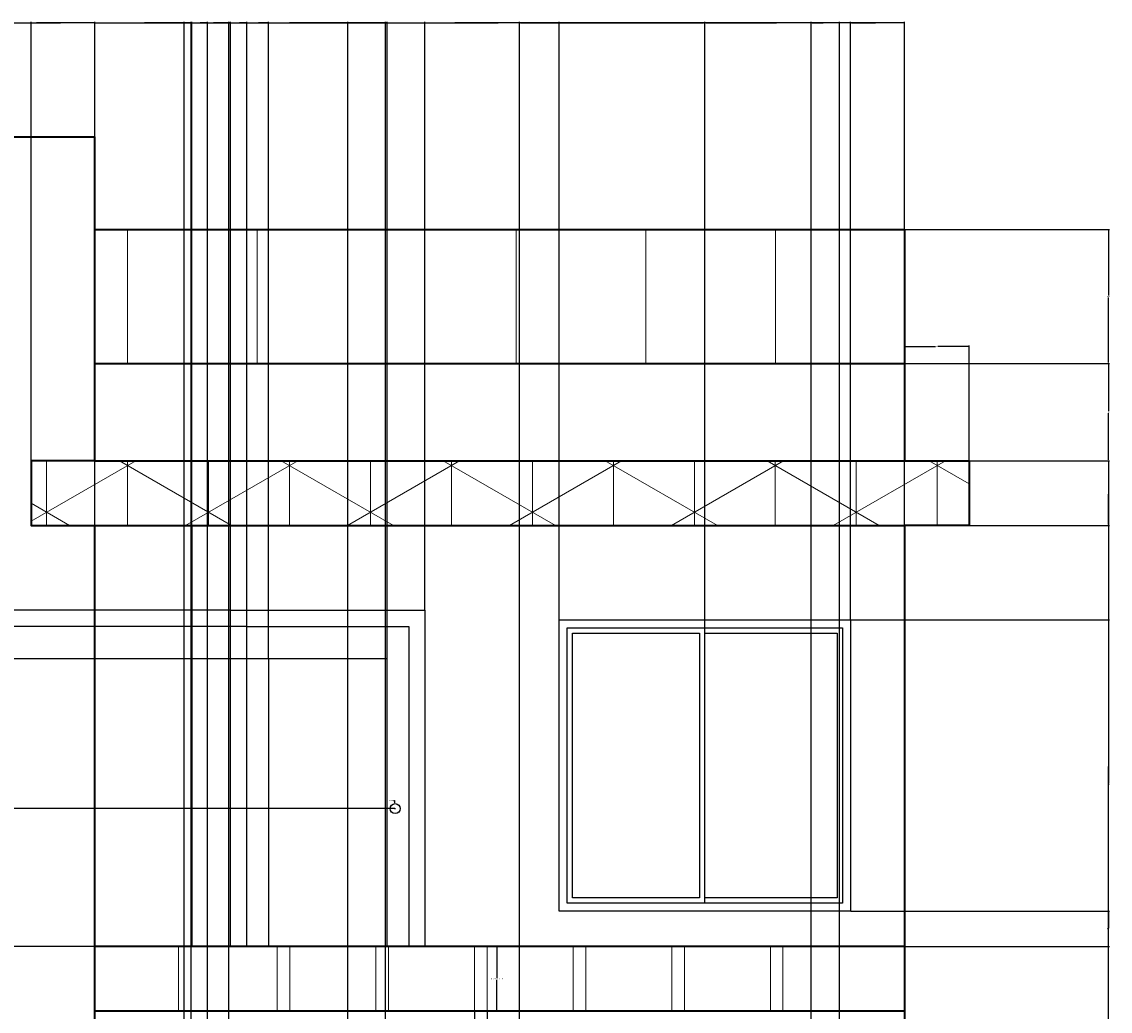
# Model space of a CAD drawing. Units: inches. Extents: x -3 to 302, y -138 to 325.
# Tile 5 of 5: x 100 to 302, y 141 to 325. Entities that reach past the tile are written whole.
import ezdxf

# ---------------------------------------------------------------- set-up
doc = ezdxf.new("R2010")
doc.units = ezdxf.units.IN
doc.header["$MEASUREMENT"] = 0
for name, color, linetype, lineweight in [('A-ANNO-DIMS', 2, 'Continuous', 18), ('A-DOOR', 4, 'Continuous', 25), ('A-ELEV', 7, 'Continuous', 35), ('A-ELEV-PATT', 8, 'Continuous', 13), ('A-ELEV-RAIL', 9, 'Continuous', 18), ('A-GLAZ', 3, 'Continuous', 25)]:
    doc.layers.add(name, color=color, linetype=linetype, lineweight=lineweight)
doc.styles.get("Standard").update_dxf_attribs({"font": 'arial.ttf'})
doc.dimstyles.get("Standard").update_dxf_attribs({"dimtxt": 0.18, "dimasz": 0.18, "dimexe": 0.18, "dimexo": 0.0625, "dimgap": 0.09, "dimtad": 0, "dimtih": 1, "dimtoh": 1, "dimdec": 4, "dimzin": 0, "dimdsep": 46, "dimtxsty": 'Standard', "dimcen": 0.09, "dimadec": 0, "dimazin": 0, "dimtfac": 1, "dimtdec": 4, "dimtofl": 0, "dimtmove": 0, "dimatfit": 3, "dimfxl": 1, "dimtolj": 1, "dimtzin": 0, "dimarcsym": 0})

# ---------------------------------------------------------------- blocks, each defined once
blk = doc.blocks.new('*U2')
for p, q in [((1.5, 1.5), (1.5, 52.5)), ((1.5, 52.5), (27, 52.5)), ((27, 1.5), (27, 52.5)), ((27, 52.5), (52.5, 52.5)), ((52.5, 52.5), (52.5, 1.5)), ((27, 1.5), (1.5, 1.5)), ((52.5, 1.5), (27, 1.5))]:
    blk.add_line(p, q)
blk.add_lwpolyline([(0, 0), (0, 54), (54, 54), (54, 0)], close=True)
for points in [[(26, 51.5), (26, 2.5), (2.5, 2.5), (2.5, 51.5), (26, 51.5)], [(27, 51.5), (51.5, 51.5), (51.5, 2.5), (27, 2.5)]]:
    blk.add_lwpolyline(points)
blk = doc.blocks.new('DOOR-FRAME-ELEV')
for points in [[(139.09, 45.37), (139.09, 107.7), (175.09, 107.7), (175.09, 45.37)], [(142.09, 45.37), (142.09, 104.67), (172.09, 104.67), (172.09, 45.37)], [(168.09, 45.37), (168.09, 98.67), (146.09, 98.67), (146.09, 45.37)]]:
    blk.add_lwpolyline(points)
blk = doc.blocks.new('RAIL-POST-2')
for p, q in [((0, 0), (0, 12)), ((2.31, 12), (2.31, 0)), ((2.31, 0), (0, 0))]:
    blk.add_line(p, q)
blk = doc.blocks.new('*D15')
at = {"layer": 'A-ANNO-DIMS', "color": 0, "lineweight": -2, "transparency": 16777216}
for p, q in [((186.67, 153.37), (188.59, 153.37)), ((188.41, 153.19), (188.41, 147.56)), ((188.41, 141.55), (188.41, 147.19)), ((186.67, 141.37), (188.59, 141.37))]:
    blk.add_line(p, q, dxfattribs=at)
at = {"layer": 'A-ANNO-DIMS', "color": 0, "transparency": 16777216}
for points in [[(188.38, 153.19), (188.44, 153.19), (188.41, 153.37)], [(188.38, 141.55), (188.44, 141.55), (188.41, 141.37)]]:
    blk.add_solid(points, dxfattribs=at)
at = {"layer": 'Defpoints', "color": 0, "transparency": 16777216}
for p in [(186.61, 153.37), (188.41, 153.37), (186.61, 141.37)]:
    blk.add_point(p, dxfattribs=at)
at = {"layer": 'A-ANNO-DIMS', "color": 0, "transparency": 16777216, "insert": (188.41, 147.37), "char_height": 0.18, "attachment_point": 5}
blk.add_mtext('\\A1;RAILING POST 12 TYP.', dxfattribs=at)
blk = doc.blocks.new('*D16')
at = {"layer": 'A-ANNO-DIMS', "color": 0, "lineweight": -2, "transparency": 16777216}
for p, q in [((184.3, 141.31), (184.3, 139.39)), ((186.61, 141.31), (186.61, 139.39)), ((184.48, 139.57), (184.99, 139.57)), ((186.43, 139.57), (185.91, 139.57))]:
    blk.add_line(p, q, dxfattribs=at)
at = {"layer": 'A-ANNO-DIMS', "color": 0, "transparency": 16777216}
for points in [[(184.48, 139.6), (184.48, 139.54), (184.3, 139.57)], [(186.43, 139.6), (186.43, 139.54), (186.61, 139.57)]]:
    blk.add_solid(points, dxfattribs=at)
at = {"layer": 'Defpoints', "color": 0, "transparency": 16777216}
for p in [(184.3, 141.37), (186.61, 141.37), (186.61, 139.57)]:
    blk.add_point(p, dxfattribs=at)
at = {"layer": 'A-ANNO-DIMS', "color": 0, "transparency": 16777216, "insert": (185.45, 139.57), "char_height": 0.18, "attachment_point": 5}
blk.add_mtext('\\A1;2 TYP.', dxfattribs=at)
blk = doc.blocks.new('*D21')
at = {"layer": 'A-ANNO-DIMS', "color": 0, "lineweight": -2, "transparency": 16777216}
for p, q in [((275.98, 243.37), (301.92, 243.37)), ((301.74, 243.19), (301.74, 183.56)), ((301.74, 123.55), (301.74, 183.19)), ((275.98, 123.37), (301.92, 123.37))]:
    blk.add_line(p, q, dxfattribs=at)
at = {"layer": 'A-ANNO-DIMS', "color": 0, "transparency": 16777216}
for points in [[(301.71, 243.19), (301.77, 243.19), (301.74, 243.37)], [(301.71, 123.55), (301.77, 123.55), (301.74, 123.37)]]:
    blk.add_solid(points, dxfattribs=at)
at = {"layer": 'Defpoints', "color": 0, "transparency": 16777216}
for p in [(275.92, 243.37), (301.74, 243.37), (275.92, 123.37)]:
    blk.add_point(p, dxfattribs=at)
at = {"layer": 'A-ANNO-DIMS', "color": 0, "transparency": 16777216, "insert": (301.74, 183.37), "char_height": 0.18, "attachment_point": 5}
blk.add_mtext('\\A1;120', dxfattribs=at)
blk = doc.blocks.new('*D22')
at = {"layer": 'A-ANNO-DIMS', "color": 0, "lineweight": -2, "transparency": 16777216}
for p, q in [((263.98, 261.37), (301.92, 261.37)), ((301.74, 261.19), (301.74, 252.56)), ((301.74, 243.55), (301.74, 252.19)), ((263.98, 243.37), (301.92, 243.37))]:
    blk.add_line(p, q, dxfattribs=at)
at = {"layer": 'A-ANNO-DIMS', "color": 0, "transparency": 16777216}
for points in [[(301.71, 261.19), (301.77, 261.19), (301.74, 261.37)], [(301.71, 243.55), (301.77, 243.55), (301.74, 243.37)]]:
    blk.add_solid(points, dxfattribs=at)
at = {"layer": 'Defpoints', "color": 0, "transparency": 16777216}
for p in [(263.92, 261.37), (301.74, 261.37), (263.92, 243.37)]:
    blk.add_point(p, dxfattribs=at)
at = {"layer": 'A-ANNO-DIMS', "color": 0, "transparency": 16777216, "insert": (301.74, 252.37), "char_height": 0.18, "attachment_point": 5}
blk.add_mtext('\\A1;18', dxfattribs=at)
blk = doc.blocks.new('*D23')
at = {"layer": 'A-ANNO-DIMS', "color": 0, "lineweight": -2, "transparency": 16777216}
for p, q in [((263.98, 286.19), (301.92, 286.19)), ((301.74, 286.01), (301.74, 273.97)), ((301.74, 261.55), (301.74, 273.6)), ((263.98, 261.37), (301.92, 261.37))]:
    blk.add_line(p, q, dxfattribs=at)
at = {"layer": 'A-ANNO-DIMS', "color": 0, "transparency": 16777216}
for points in [[(301.71, 286.01), (301.77, 286.01), (301.74, 286.19)], [(301.71, 261.55), (301.77, 261.55), (301.74, 261.37)]]:
    blk.add_solid(points, dxfattribs=at)
at = {"layer": 'Defpoints', "color": 0, "transparency": 16777216}
for p in [(263.92, 286.19), (301.74, 286.19), (263.92, 261.37)]:
    blk.add_point(p, dxfattribs=at)
at = {"layer": 'A-ANNO-DIMS', "color": 0, "transparency": 16777216, "insert": (301.74, 273.78), "char_height": 0.18, "attachment_point": 5}
blk.add_mtext('\\A1;24.82', dxfattribs=at)
blk = doc.blocks.new('*D27')
at = {"layer": 'A-ANNO-DIMS', "color": 0, "lineweight": -2, "transparency": 16777216}
for p, q in [((91.92, 245.44), (91.92, 324.7)), ((113.92, 303.44), (113.92, 324.7)), ((92.1, 324.52), (102.7, 324.52)), ((113.74, 324.52), (103.14, 324.52))]:
    blk.add_line(p, q, dxfattribs=at)
at = {"layer": 'A-ANNO-DIMS', "color": 0, "transparency": 16777216}
for points in [[(92.1, 324.55), (92.1, 324.49), (91.92, 324.52)], [(113.74, 324.55), (113.74, 324.49), (113.92, 324.52)]]:
    blk.add_solid(points, dxfattribs=at)
at = {"layer": 'Defpoints', "color": 0, "transparency": 16777216}
for p in [(113.92, 324.52), (113.92, 303.37), (91.92, 245.37)]:
    blk.add_point(p, dxfattribs=at)
at = {"layer": 'A-ANNO-DIMS', "color": 0, "transparency": 16777216, "insert": (102.92, 324.52), "char_height": 0.18, "attachment_point": 5}
blk.add_mtext('\\A1;22', dxfattribs=at)
blk = doc.blocks.new('*D28')
at = {"layer": 'A-ANNO-DIMS', "color": 0, "lineweight": -2, "transparency": 16777216}
for p, q in [((113.92, 286.26), (113.92, 324.7)), ((263.92, 286.26), (263.92, 324.7)), ((114.1, 324.52), (188.64, 324.52)), ((263.74, 324.52), (189.2, 324.52))]:
    blk.add_line(p, q, dxfattribs=at)
at = {"layer": 'A-ANNO-DIMS', "color": 0, "transparency": 16777216}
for points in [[(114.1, 324.55), (114.1, 324.49), (113.92, 324.52)], [(263.74, 324.55), (263.74, 324.49), (263.92, 324.52)]]:
    blk.add_solid(points, dxfattribs=at)
at = {"layer": 'Defpoints', "color": 0, "transparency": 16777216}
for p in [(263.92, 324.52), (113.92, 286.19), (263.92, 286.19)]:
    blk.add_point(p, dxfattribs=at)
at = {"layer": 'A-ANNO-DIMS', "color": 0, "transparency": 16777216, "insert": (188.92, 324.52), "char_height": 0.18, "attachment_point": 5}
blk.add_mtext('\\A1;150', dxfattribs=at)
blk = doc.blocks.new('*D29')
at = {"layer": 'A-ANNO-DIMS', "color": 0, "lineweight": -2, "transparency": 16777216}
for p, q in [((263.92, 243.44), (263.92, 264.7)), ((264.1, 264.52), (269.71, 264.52)), ((275.74, 264.52), (270.13, 264.52)), ((275.92, 243.44), (275.92, 264.7))]:
    blk.add_line(p, q, dxfattribs=at)
at = {"layer": 'A-ANNO-DIMS', "color": 0, "transparency": 16777216}
for points in [[(264.1, 264.55), (264.1, 264.49), (263.92, 264.52)], [(275.74, 264.55), (275.74, 264.49), (275.92, 264.52)]]:
    blk.add_solid(points, dxfattribs=at)
at = {"layer": 'Defpoints', "color": 0, "transparency": 16777216}
for p in [(275.92, 264.52), (263.92, 243.37), (275.92, 243.37)]:
    blk.add_point(p, dxfattribs=at)
at = {"layer": 'A-ANNO-DIMS', "color": 0, "transparency": 16777216, "insert": (269.92, 264.52), "char_height": 0.18, "attachment_point": 5}
blk.add_mtext('\\A1;12', dxfattribs=at)
blk = doc.blocks.new('*D30')
at = {"layer": 'A-ANNO-DIMS', "color": 0, "lineweight": -2, "transparency": 16777216}
for p, q in [((102.13, 243.44), (102.13, 324.7)), ((113.92, 243.44), (113.92, 324.7)), ((102.31, 324.52), (107.57, 324.52)), ((113.74, 324.52), (108.48, 324.52))]:
    blk.add_line(p, q, dxfattribs=at)
at = {"layer": 'A-ANNO-DIMS', "color": 0, "transparency": 16777216}
for points in [[(102.31, 324.55), (102.31, 324.49), (102.13, 324.52)], [(113.74, 324.55), (113.74, 324.49), (113.92, 324.52)]]:
    blk.add_solid(points, dxfattribs=at)
at = {"layer": 'Defpoints', "color": 0, "transparency": 16777216}
for p in [(113.92, 324.52), (102.13, 243.37), (113.92, 243.37)]:
    blk.add_point(p, dxfattribs=at)
at = {"layer": 'A-ANNO-DIMS', "color": 0, "transparency": 16777216, "insert": (108.03, 324.52), "char_height": 0.18, "attachment_point": 5}
blk.add_mtext('\\A1;11.787', dxfattribs=at)
blk = doc.blocks.new('*D39')
at = {"layer": 'A-ANNO-DIMS', "color": 0, "lineweight": -2, "transparency": 16777216}
for p, q in [((275.98, 243.37), (301.92, 243.37)), ((301.74, 243.19), (301.74, 237.56)), ((301.74, 231.55), (301.74, 237.19)), ((275.98, 231.37), (301.92, 231.37))]:
    blk.add_line(p, q, dxfattribs=at)
at = {"layer": 'A-ANNO-DIMS', "color": 0, "transparency": 16777216}
for points in [[(301.71, 243.19), (301.77, 243.19), (301.74, 243.37)], [(301.71, 231.55), (301.77, 231.55), (301.74, 231.37)]]:
    blk.add_solid(points, dxfattribs=at)
at = {"layer": 'Defpoints', "color": 0, "transparency": 16777216}
for p in [(275.92, 243.37), (301.74, 243.37), (275.92, 231.37)]:
    blk.add_point(p, dxfattribs=at)
at = {"layer": 'A-ANNO-DIMS', "color": 0, "transparency": 16777216, "insert": (301.74, 237.37), "char_height": 0.18, "attachment_point": 5}
blk.add_mtext('\\A1;12', dxfattribs=at)
blk = doc.blocks.new('*D50')
at = {"layer": 'A-ANNO-DIMS', "color": 0, "lineweight": -2, "transparency": 16777216}
for p, q in [((113.92, 153.44), (113.92, 324.7)), ((131.92, 153.44), (131.92, 324.7)), ((114.1, 324.52), (122.71, 324.52)), ((131.74, 324.52), (123.13, 324.52))]:
    blk.add_line(p, q, dxfattribs=at)
at = {"layer": 'A-ANNO-DIMS', "color": 0, "transparency": 16777216}
for points in [[(114.1, 324.55), (114.1, 324.49), (113.92, 324.52)], [(131.74, 324.55), (131.74, 324.49), (131.92, 324.52)]]:
    blk.add_solid(points, dxfattribs=at)
at = {"layer": 'Defpoints', "color": 0, "transparency": 16777216}
for p in [(131.92, 324.52), (113.92, 153.37), (131.92, 153.37)]:
    blk.add_point(p, dxfattribs=at)
at = {"layer": 'A-ANNO-DIMS', "color": 0, "transparency": 16777216, "insert": (122.92, 324.52), "char_height": 0.18, "attachment_point": 5}
blk.add_mtext('\\A1;18', dxfattribs=at)
blk = doc.blocks.new('*D51')
at = {"layer": 'A-ANNO-DIMS', "color": 0, "lineweight": -2, "transparency": 16777216}
for p, q in [((131.92, 153.44), (131.92, 324.7)), ((139.09, 215.76), (139.09, 324.7)), ((132.1, 324.52), (135.11, 324.52)), ((138.91, 324.52), (135.9, 324.52))]:
    blk.add_line(p, q, dxfattribs=at)
at = {"layer": 'A-ANNO-DIMS', "color": 0, "transparency": 16777216}
for points in [[(132.1, 324.55), (132.1, 324.49), (131.92, 324.52)], [(138.91, 324.55), (138.91, 324.49), (139.09, 324.52)]]:
    blk.add_solid(points, dxfattribs=at)
at = {"layer": 'Defpoints', "color": 0, "transparency": 16777216}
for p in [(139.09, 324.52), (139.09, 215.7), (131.92, 153.37)]:
    blk.add_point(p, dxfattribs=at)
at = {"layer": 'A-ANNO-DIMS', "color": 0, "transparency": 16777216, "insert": (135.5, 324.52), "char_height": 0.18, "attachment_point": 5}
blk.add_mtext('\\A1;7.164', dxfattribs=at)
blk = doc.blocks.new('*D52')
at = {"layer": 'A-ANNO-DIMS', "color": 0, "lineweight": -2, "transparency": 16777216}
for p, q in [((175.09, 215.76), (175.09, 324.7)), ((199.94, 213.98), (199.94, 324.7)), ((175.27, 324.52), (187.12, 324.52)), ((199.76, 324.52), (187.91, 324.52))]:
    blk.add_line(p, q, dxfattribs=at)
at = {"layer": 'A-ANNO-DIMS', "color": 0, "transparency": 16777216}
for points in [[(175.27, 324.55), (175.27, 324.49), (175.09, 324.52)], [(199.76, 324.55), (199.76, 324.49), (199.94, 324.52)]]:
    blk.add_solid(points, dxfattribs=at)
at = {"layer": 'Defpoints', "color": 0, "transparency": 16777216}
for p in [(199.94, 324.52), (175.09, 215.7), (199.94, 213.91)]:
    blk.add_point(p, dxfattribs=at)
at = {"layer": 'A-ANNO-DIMS', "color": 0, "transparency": 16777216, "insert": (187.51, 324.52), "char_height": 0.18, "attachment_point": 5}
blk.add_mtext('\\A1;24.85', dxfattribs=at)
blk = doc.blocks.new('*D53')
at = {"layer": 'A-ANNO-DIMS', "color": 0, "lineweight": -2, "transparency": 16777216}
for p, q in [((199.94, 213.98), (199.94, 324.7)), ((253.94, 213.98), (253.94, 324.7)), ((200.12, 324.52), (226.72, 324.52)), ((253.76, 324.52), (227.15, 324.52))]:
    blk.add_line(p, q, dxfattribs=at)
at = {"layer": 'A-ANNO-DIMS', "color": 0, "transparency": 16777216}
for points in [[(200.12, 324.55), (200.12, 324.49), (199.94, 324.52)], [(253.76, 324.55), (253.76, 324.49), (253.94, 324.52)]]:
    blk.add_solid(points, dxfattribs=at)
at = {"layer": 'Defpoints', "color": 0, "transparency": 16777216}
for p in [(253.94, 324.52), (199.94, 213.91), (253.94, 213.91)]:
    blk.add_point(p, dxfattribs=at)
at = {"layer": 'A-ANNO-DIMS', "color": 0, "transparency": 16777216, "insert": (226.94, 324.52), "char_height": 0.18, "attachment_point": 5}
blk.add_mtext('\\A1;54', dxfattribs=at)
blk = doc.blocks.new('*D54')
at = {"layer": 'A-ANNO-DIMS', "color": 0, "lineweight": -2, "transparency": 16777216}
for p, q in [((253.94, 213.98), (253.94, 324.7)), ((263.92, 153.44), (263.92, 324.7)), ((254.12, 324.52), (258.54, 324.52)), ((263.74, 324.52), (259.32, 324.52))]:
    blk.add_line(p, q, dxfattribs=at)
at = {"layer": 'A-ANNO-DIMS', "color": 0, "transparency": 16777216}
for points in [[(254.12, 324.55), (254.12, 324.49), (253.94, 324.52)], [(263.74, 324.55), (263.74, 324.49), (263.92, 324.52)]]:
    blk.add_solid(points, dxfattribs=at)
at = {"layer": 'Defpoints', "color": 0, "transparency": 16777216}
for p in [(263.92, 324.52), (253.94, 213.91), (263.92, 153.37)]:
    blk.add_point(p, dxfattribs=at)
at = {"layer": 'A-ANNO-DIMS', "color": 0, "transparency": 16777216, "insert": (258.93, 324.52), "char_height": 0.18, "attachment_point": 5}
blk.add_mtext('\\A1;9.986', dxfattribs=at)
blk = doc.blocks.new('*D55')
at = {"layer": 'A-ANNO-DIMS', "color": 0, "lineweight": -2, "transparency": 16777216}
for p, q in [((139.09, 215.76), (139.09, 324.7)), ((142.09, 212.74), (142.09, 324.7)), ((139.27, 324.52), (140.44, 324.52)), ((141.91, 324.52), (140.74, 324.52))]:
    blk.add_line(p, q, dxfattribs=at)
at = {"layer": 'A-ANNO-DIMS', "color": 0, "transparency": 16777216}
for points in [[(139.27, 324.55), (139.27, 324.49), (139.09, 324.52)], [(141.91, 324.55), (141.91, 324.49), (142.09, 324.52)]]:
    blk.add_solid(points, dxfattribs=at)
at = {"layer": 'Defpoints', "color": 0, "transparency": 16777216}
for p in [(142.09, 324.52), (139.09, 215.7), (142.09, 212.67)]:
    blk.add_point(p, dxfattribs=at)
at = {"layer": 'A-ANNO-DIMS', "color": 0, "transparency": 16777216, "insert": (140.59, 324.52), "char_height": 0.18, "attachment_point": 5}
blk.add_mtext('\\A1;3', dxfattribs=at)
blk = doc.blocks.new('*D56')
at = {"layer": 'A-ANNO-DIMS', "color": 0, "lineweight": -2, "transparency": 16777216}
for p, q in [((142.09, 212.74), (142.09, 324.7)), ((146.09, 206.74), (146.09, 324.7)), ((142.27, 324.52), (143.93, 324.52)), ((145.91, 324.52), (144.24, 324.52))]:
    blk.add_line(p, q, dxfattribs=at)
at = {"layer": 'A-ANNO-DIMS', "color": 0, "transparency": 16777216}
for points in [[(142.27, 324.55), (142.27, 324.49), (142.09, 324.52)], [(145.91, 324.55), (145.91, 324.49), (146.09, 324.52)]]:
    blk.add_solid(points, dxfattribs=at)
at = {"layer": 'Defpoints', "color": 0, "transparency": 16777216}
for p in [(146.09, 324.52), (142.09, 212.67), (146.09, 206.67)]:
    blk.add_point(p, dxfattribs=at)
at = {"layer": 'A-ANNO-DIMS', "color": 0, "transparency": 16777216, "insert": (144.09, 324.52), "char_height": 0.18, "attachment_point": 5}
blk.add_mtext('\\A1;4', dxfattribs=at)
blk = doc.blocks.new('*D57')
at = {"layer": 'A-ANNO-DIMS', "color": 0, "lineweight": -2, "transparency": 16777216}
for p, q in [((146.09, 206.74), (146.09, 324.7)), ((168.09, 206.74), (168.09, 324.7)), ((146.27, 324.52), (156.87, 324.52)), ((167.91, 324.52), (157.31, 324.52))]:
    blk.add_line(p, q, dxfattribs=at)
at = {"layer": 'A-ANNO-DIMS', "color": 0, "transparency": 16777216}
for points in [[(146.27, 324.55), (146.27, 324.49), (146.09, 324.52)], [(167.91, 324.55), (167.91, 324.49), (168.09, 324.52)]]:
    blk.add_solid(points, dxfattribs=at)
at = {"layer": 'Defpoints', "color": 0, "transparency": 16777216}
for p in [(168.09, 324.52), (146.09, 206.67), (168.09, 206.67)]:
    blk.add_point(p, dxfattribs=at)
at = {"layer": 'A-ANNO-DIMS', "color": 0, "transparency": 16777216, "insert": (157.09, 324.52), "char_height": 0.18, "attachment_point": 5}
blk.add_mtext('\\A1;22', dxfattribs=at)
blk = doc.blocks.new('*D58')
at = {"layer": 'A-ANNO-DIMS', "color": 0, "lineweight": -2, "transparency": 16777216}
for p, q in [((199.94, 213.98), (199.94, 324.7)), ((226.94, 212.48), (226.94, 324.7)), ((200.12, 324.52), (213.22, 324.52)), ((226.76, 324.52), (213.66, 324.52))]:
    blk.add_line(p, q, dxfattribs=at)
at = {"layer": 'A-ANNO-DIMS', "color": 0, "transparency": 16777216}
for points in [[(200.12, 324.55), (200.12, 324.49), (199.94, 324.52)], [(226.76, 324.55), (226.76, 324.49), (226.94, 324.52)]]:
    blk.add_solid(points, dxfattribs=at)
at = {"layer": 'Defpoints', "color": 0, "transparency": 16777216}
for p in [(226.94, 324.52), (199.94, 213.91), (226.94, 212.41)]:
    blk.add_point(p, dxfattribs=at)
at = {"layer": 'A-ANNO-DIMS', "color": 0, "transparency": 16777216, "insert": (213.44, 324.52), "char_height": 0.18, "attachment_point": 5}
blk.add_mtext('\\A1;27', dxfattribs=at)
blk = doc.blocks.new('*D59')
at = {"layer": 'A-ANNO-DIMS', "color": 0, "lineweight": -2, "transparency": 16777216}
for p, q in [((226.94, 212.48), (226.94, 324.7)), ((253.94, 213.98), (253.94, 324.7)), ((227.12, 324.52), (240.22, 324.52)), ((253.76, 324.52), (240.66, 324.52))]:
    blk.add_line(p, q, dxfattribs=at)
at = {"layer": 'A-ANNO-DIMS', "color": 0, "transparency": 16777216}
for points in [[(227.12, 324.55), (227.12, 324.49), (226.94, 324.52)], [(253.76, 324.55), (253.76, 324.49), (253.94, 324.52)]]:
    blk.add_solid(points, dxfattribs=at)
at = {"layer": 'Defpoints', "color": 0, "transparency": 16777216}
for p in [(253.94, 324.52), (253.94, 213.91), (226.94, 212.41)]:
    blk.add_point(p, dxfattribs=at)
at = {"layer": 'A-ANNO-DIMS', "color": 0, "transparency": 16777216, "insert": (240.44, 324.52), "char_height": 0.18, "attachment_point": 5}
blk.add_mtext('\\A1;27', dxfattribs=at)
blk = doc.blocks.new('*D60')
at = {"layer": 'A-ANNO-DIMS', "color": 0, "lineweight": -2, "transparency": 16777216}
for p, q in [((146.02, 206.67), (-2.8, 206.67)), ((-2.62, 206.49), (-2.62, 180.21)), ((-2.62, 153.55), (-2.62, 179.84)), ((139.02, 153.37), (-2.8, 153.37))]:
    blk.add_line(p, q, dxfattribs=at)
at = {"layer": 'A-ANNO-DIMS', "color": 0, "transparency": 16777216}
for points in [[(-2.65, 206.49), (-2.59, 206.49), (-2.62, 206.67)], [(-2.65, 153.55), (-2.59, 153.55), (-2.62, 153.37)]]:
    blk.add_solid(points, dxfattribs=at)
at = {"layer": 'Defpoints', "color": 0, "transparency": 16777216}
for p in [(-2.62, 206.67), (146.09, 206.67), (139.09, 153.37)]:
    blk.add_point(p, dxfattribs=at)
at = {"layer": 'A-ANNO-DIMS', "color": 0, "transparency": 16777216, "insert": (-2.62, 180.02), "char_height": 0.18, "attachment_point": 5}
blk.add_mtext('\\A1;53.3', dxfattribs=at)
blk = doc.blocks.new('*D61')
at = {"layer": 'A-ANNO-DIMS', "color": 0, "lineweight": -2, "transparency": 16777216}
for p, q in [((142.02, 212.67), (-2.8, 212.67)), ((-2.62, 212.49), (-2.62, 209.86)), ((-2.62, 206.85), (-2.62, 209.49)), ((146.02, 206.67), (-2.8, 206.67))]:
    blk.add_line(p, q, dxfattribs=at)
at = {"layer": 'A-ANNO-DIMS', "color": 0, "transparency": 16777216}
for points in [[(-2.65, 212.49), (-2.59, 212.49), (-2.62, 212.67)], [(-2.65, 206.85), (-2.59, 206.85), (-2.62, 206.67)]]:
    blk.add_solid(points, dxfattribs=at)
at = {"layer": 'Defpoints', "color": 0, "transparency": 16777216}
for p in [(-2.62, 212.67), (142.09, 212.67), (146.09, 206.67)]:
    blk.add_point(p, dxfattribs=at)
at = {"layer": 'A-ANNO-DIMS', "color": 0, "transparency": 16777216, "insert": (-2.62, 209.67), "char_height": 0.18, "attachment_point": 5}
blk.add_mtext('\\A1;6', dxfattribs=at)
blk = doc.blocks.new('*D62')
at = {"layer": 'A-ANNO-DIMS', "color": 0, "lineweight": -2, "transparency": 16777216}
for p, q in [((139.02, 215.7), (-2.8, 215.7)), ((-2.62, 215.52), (-2.62, 214.37)), ((-2.62, 212.85), (-2.62, 214)), ((142.02, 212.67), (-2.8, 212.67))]:
    blk.add_line(p, q, dxfattribs=at)
at = {"layer": 'A-ANNO-DIMS', "color": 0, "transparency": 16777216}
for points in [[(-2.65, 215.52), (-2.59, 215.52), (-2.62, 215.7)], [(-2.65, 212.85), (-2.59, 212.85), (-2.62, 212.67)]]:
    blk.add_solid(points, dxfattribs=at)
at = {"layer": 'Defpoints', "color": 0, "transparency": 16777216}
for p in [(-2.62, 215.7), (139.09, 215.7), (142.09, 212.67)]:
    blk.add_point(p, dxfattribs=at)
at = {"layer": 'A-ANNO-DIMS', "color": 0, "transparency": 16777216, "insert": (-2.62, 214.19), "char_height": 0.18, "attachment_point": 5}
blk.add_mtext('\\A1;3.023', dxfattribs=at)
blk = doc.blocks.new('*D63')
at = {"layer": 'A-ANNO-DIMS', "color": 0, "lineweight": -2, "transparency": 16777216}
for p, q in [((169.52, 178.91), (-2.8, 178.91)), ((-2.62, 178.73), (-2.62, 166.33)), ((-2.62, 153.55), (-2.62, 165.96)), ((168.02, 153.37), (-2.8, 153.37))]:
    blk.add_line(p, q, dxfattribs=at)
at = {"layer": 'A-ANNO-DIMS', "color": 0, "transparency": 16777216}
for points in [[(-2.65, 178.73), (-2.59, 178.73), (-2.62, 178.91)], [(-2.65, 153.55), (-2.59, 153.55), (-2.62, 153.37)]]:
    blk.add_solid(points, dxfattribs=at)
at = {"layer": 'Defpoints', "color": 0, "transparency": 16777216}
for p in [(-2.62, 178.91), (169.58, 178.91), (168.09, 153.37)]:
    blk.add_point(p, dxfattribs=at)
at = {"layer": 'A-ANNO-DIMS', "color": 0, "transparency": 16777216, "insert": (-2.62, 166.14), "char_height": 0.18, "attachment_point": 5}
blk.add_mtext('\\A1;25.54', dxfattribs=at)
blk = doc.blocks.new('*D64')
at = {"layer": 'A-ANNO-DIMS', "color": 0, "lineweight": -2, "transparency": 16777216}
for p, q in [((254, 159.91), (301.92, 159.91)), ((301.74, 159.73), (301.74, 156.83)), ((301.74, 153.55), (301.74, 156.46)), ((263.98, 153.37), (301.92, 153.37))]:
    blk.add_line(p, q, dxfattribs=at)
at = {"layer": 'A-ANNO-DIMS', "color": 0, "transparency": 16777216}
for points in [[(301.71, 159.73), (301.77, 159.73), (301.74, 159.91)], [(301.71, 153.55), (301.77, 153.55), (301.74, 153.37)]]:
    blk.add_solid(points, dxfattribs=at)
at = {"layer": 'Defpoints', "color": 0, "transparency": 16777216}
for p in [(253.94, 159.91), (301.74, 159.91), (263.92, 153.37)]:
    blk.add_point(p, dxfattribs=at)
at = {"layer": 'A-ANNO-DIMS', "color": 0, "transparency": 16777216, "insert": (301.74, 156.64), "char_height": 0.18, "attachment_point": 5}
blk.add_mtext('\\A1;6.539', dxfattribs=at)
blk = doc.blocks.new('*D65')
at = {"layer": 'A-ANNO-DIMS', "color": 0, "lineweight": -2, "transparency": 16777216}
for p, q in [((254, 213.91), (301.92, 213.91)), ((301.74, 213.73), (301.74, 187.1)), ((301.74, 160.09), (301.74, 186.73)), ((254, 159.91), (301.92, 159.91))]:
    blk.add_line(p, q, dxfattribs=at)
at = {"layer": 'A-ANNO-DIMS', "color": 0, "transparency": 16777216}
for points in [[(301.71, 213.73), (301.77, 213.73), (301.74, 213.91)], [(301.71, 160.09), (301.77, 160.09), (301.74, 159.91)]]:
    blk.add_solid(points, dxfattribs=at)
at = {"layer": 'Defpoints', "color": 0, "transparency": 16777216}
for p in [(253.94, 213.91), (301.74, 213.91), (253.94, 159.91)]:
    blk.add_point(p, dxfattribs=at)
at = {"layer": 'A-ANNO-DIMS', "color": 0, "transparency": 16777216, "insert": (301.74, 186.91), "char_height": 0.18, "attachment_point": 5}
blk.add_mtext('\\A1;54', dxfattribs=at)
blk = doc.blocks.new('*D68')
at = {"layer": 'A-ANNO-DIMS', "color": 0, "lineweight": -2, "transparency": 16777216}
for p, q in [((130.489456, -43.793388), (130.489456, 324.704711)), ((131.787096, -26.240874), (131.787096, 324.704711)), ((130.669456, 324.524711), (130.823276, 324.524711)), ((131.607096, 324.524711), (131.453276, 324.524711))]:
    blk.add_line(p, q, dxfattribs=at)
at = {"layer": 'A-ANNO-DIMS', "color": 0, "transparency": 16777216}
for points in [[(130.669456, 324.554711), (130.669456, 324.494711), (130.489456, 324.524711)], [(131.607096, 324.554711), (131.607096, 324.494711), (131.787096, 324.524711)]]:
    blk.add_solid(points, dxfattribs=at)
at = {"layer": 'Defpoints', "color": 0, "transparency": 16777216}
for p in [(131.787096, 324.524711), (131.787096, -26.303374), (130.489456, -43.855888)]:
    blk.add_point(p, dxfattribs=at)
at = {"layer": 'A-ANNO-DIMS', "color": 0, "transparency": 16777216, "insert": (131.138276, 324.524711), "char_height": 0.18, "attachment_point": 5}
blk.add_mtext('\\A1;1.30', dxfattribs=at)
blk = doc.blocks.new('*D69')
at = {"layer": 'A-ANNO-DIMS', "color": 0, "lineweight": -2, "transparency": 16777216}
for p, q in [((131.79, -26.24), (131.79, 324.7)), ((167.79, -26.24), (167.79, 324.7)), ((131.97, 324.52), (149.57, 324.52)), ((167.61, 324.52), (150.01, 324.52))]:
    blk.add_line(p, q, dxfattribs=at)
at = {"layer": 'A-ANNO-DIMS', "color": 0, "transparency": 16777216}
for points in [[(131.97, 324.55), (131.97, 324.49), (131.79, 324.52)], [(167.61, 324.55), (167.61, 324.49), (167.79, 324.52)]]:
    blk.add_solid(points, dxfattribs=at)
at = {"layer": 'Defpoints', "color": 0, "transparency": 16777216}
for p in [(167.79, 324.52), (131.79, -26.3), (167.79, -26.3)]:
    blk.add_point(p, dxfattribs=at)
at = {"layer": 'A-ANNO-DIMS', "color": 0, "transparency": 16777216, "insert": (149.79, 324.52), "char_height": 0.18, "attachment_point": 5}
blk.add_mtext('\\A1;36', dxfattribs=at)
blk = doc.blocks.new('*D70')
at = {"layer": 'A-ANNO-DIMS', "color": 0, "lineweight": -2, "transparency": 16777216}
for p, q in [((167.79, -26.24), (167.79, 324.7)), ((192.64, -28.02), (192.64, 324.7)), ((167.97, 324.52), (179.82, 324.52)), ((192.46, 324.52), (180.61, 324.52))]:
    blk.add_line(p, q, dxfattribs=at)
at = {"layer": 'A-ANNO-DIMS', "color": 0, "transparency": 16777216}
for points in [[(167.97, 324.55), (167.97, 324.49), (167.79, 324.52)], [(192.46, 324.55), (192.46, 324.49), (192.64, 324.52)]]:
    blk.add_solid(points, dxfattribs=at)
at = {"layer": 'Defpoints', "color": 0, "transparency": 16777216}
for p in [(192.64, 324.52), (167.79, -26.3), (192.64, -28.09)]:
    blk.add_point(p, dxfattribs=at)
at = {"layer": 'A-ANNO-DIMS', "color": 0, "transparency": 16777216, "insert": (180.21, 324.52), "char_height": 0.18, "attachment_point": 5}
blk.add_mtext('\\A1;24.85', dxfattribs=at)
blk = doc.blocks.new('*D71')
at = {"layer": 'A-ANNO-DIMS', "color": 0, "lineweight": -2, "transparency": 16777216}
for p, q in [((192.64, -28.02), (192.64, 324.7)), ((246.64, -28.02), (246.64, 324.7)), ((192.82, 324.52), (219.42, 324.52)), ((246.46, 324.52), (219.86, 324.52))]:
    blk.add_line(p, q, dxfattribs=at)
at = {"layer": 'A-ANNO-DIMS', "color": 0, "transparency": 16777216}
for points in [[(192.82, 324.55), (192.82, 324.49), (192.64, 324.52)], [(246.46, 324.55), (246.46, 324.49), (246.64, 324.52)]]:
    blk.add_solid(points, dxfattribs=at)
at = {"layer": 'Defpoints', "color": 0, "transparency": 16777216}
for p in [(246.64, 324.52), (192.64, -28.09), (246.64, -28.09)]:
    blk.add_point(p, dxfattribs=at)
at = {"layer": 'A-ANNO-DIMS', "color": 0, "transparency": 16777216, "insert": (219.64, 324.52), "char_height": 0.18, "attachment_point": 5}
blk.add_mtext('\\A1;54', dxfattribs=at)
blk = doc.blocks.new('*D72')
at = {"layer": 'A-ANNO-DIMS', "color": 0, "lineweight": -2, "transparency": 16777216}
for p, q in [((246.64, -28.02), (246.64, 324.7)), ((251.92, -49.03), (251.92, 324.7)), ((246.82, 324.52), (248.89, 324.52)), ((251.74, 324.52), (249.67, 324.52))]:
    blk.add_line(p, q, dxfattribs=at)
at = {"layer": 'A-ANNO-DIMS', "color": 0, "transparency": 16777216}
for points in [[(246.82, 324.55), (246.82, 324.49), (246.64, 324.52)], [(251.74, 324.55), (251.74, 324.49), (251.92, 324.52)]]:
    blk.add_solid(points, dxfattribs=at)
at = {"layer": 'Defpoints', "color": 0, "transparency": 16777216}
for p in [(251.92, 324.52), (246.64, -28.09), (251.92, -49.09)]:
    blk.add_point(p, dxfattribs=at)
at = {"layer": 'A-ANNO-DIMS', "color": 0, "transparency": 16777216, "insert": (249.28, 324.52), "char_height": 0.18, "attachment_point": 5}
blk.add_mtext('\\A1;5.285', dxfattribs=at)
blk = doc.blocks.new('*D73')
at = {"layer": 'A-ANNO-DIMS', "color": 0, "lineweight": -2, "transparency": 16777216}
for p, q in [((131.79, -26.24), (131.79, 324.7)), ((134.79, -29.26), (134.79, 324.7)), ((131.97, 324.52), (133.14, 324.52)), ((134.61, 324.52), (133.44, 324.52))]:
    blk.add_line(p, q, dxfattribs=at)
at = {"layer": 'A-ANNO-DIMS', "color": 0, "transparency": 16777216}
for points in [[(131.97, 324.55), (131.97, 324.49), (131.79, 324.52)], [(134.61, 324.55), (134.61, 324.49), (134.79, 324.52)]]:
    blk.add_solid(points, dxfattribs=at)
at = {"layer": 'Defpoints', "color": 0, "transparency": 16777216}
for p in [(134.79, 324.52), (131.79, -26.3), (134.79, -29.33)]:
    blk.add_point(p, dxfattribs=at)
at = {"layer": 'A-ANNO-DIMS', "color": 0, "transparency": 16777216, "insert": (133.29, 324.52), "char_height": 0.18, "attachment_point": 5}
blk.add_mtext('\\A1;3', dxfattribs=at)
blk = doc.blocks.new('*D74')
at = {"layer": 'A-ANNO-DIMS', "color": 0, "lineweight": -2, "transparency": 16777216}
for p, q in [((134.79, -29.26), (134.79, 324.7)), ((138.79, -35.26), (138.79, 324.7)), ((134.97, 324.52), (136.63, 324.52)), ((138.61, 324.52), (136.94, 324.52))]:
    blk.add_line(p, q, dxfattribs=at)
at = {"layer": 'A-ANNO-DIMS', "color": 0, "transparency": 16777216}
for points in [[(134.97, 324.55), (134.97, 324.49), (134.79, 324.52)], [(138.61, 324.55), (138.61, 324.49), (138.79, 324.52)]]:
    blk.add_solid(points, dxfattribs=at)
at = {"layer": 'Defpoints', "color": 0, "transparency": 16777216}
for p in [(138.79, 324.52), (134.79, -29.33), (138.79, -35.33)]:
    blk.add_point(p, dxfattribs=at)
at = {"layer": 'A-ANNO-DIMS', "color": 0, "transparency": 16777216, "insert": (136.79, 324.52), "char_height": 0.18, "attachment_point": 5}
blk.add_mtext('\\A1;4', dxfattribs=at)
blk = doc.blocks.new('*D75')
at = {"layer": 'A-ANNO-DIMS', "color": 0, "lineweight": -2, "transparency": 16777216}
for p, q in [((138.79, -35.26), (138.79, 324.7)), ((160.79, -35.26), (160.79, 324.7)), ((138.97, 324.52), (149.57, 324.52)), ((160.61, 324.52), (150.01, 324.52))]:
    blk.add_line(p, q, dxfattribs=at)
at = {"layer": 'A-ANNO-DIMS', "color": 0, "transparency": 16777216}
for points in [[(138.97, 324.55), (138.97, 324.49), (138.79, 324.52)], [(160.61, 324.55), (160.61, 324.49), (160.79, 324.52)]]:
    blk.add_solid(points, dxfattribs=at)
at = {"layer": 'Defpoints', "color": 0, "transparency": 16777216}
for p in [(160.79, 324.52), (138.79, -35.33), (160.79, -35.33)]:
    blk.add_point(p, dxfattribs=at)
at = {"layer": 'A-ANNO-DIMS', "color": 0, "transparency": 16777216, "insert": (149.79, 324.52), "char_height": 0.18, "attachment_point": 5}
blk.add_mtext('\\A1;22', dxfattribs=at)
blk = doc.blocks.new('*D89')
at = {"layer": 'A-ANNO-DIMS', "color": 0, "lineweight": -2, "transparency": 16777216}
for p, q in [((169.27, 180.39), (169.45, 180.39)), ((169.45, 180.39), (169.48, 180.01)), ((169.49, 178.91), (169.67, 178.91)), ((169.58, 178.82), (169.58, 179))]:
    blk.add_line(p, q, dxfattribs=at)
at = {"layer": 'A-ANNO-DIMS', "color": 0, "transparency": 16777216}
blk.add_solid([(169.51, 180.02), (169.45, 180.01), (169.5, 179.83)], dxfattribs=at)
at = {"layer": 'Defpoints', "color": 0, "transparency": 16777216}
for p in [(169.5, 179.83), (169.67, 177.99)]:
    blk.add_point(p, dxfattribs=at)
at = {"layer": 'A-ANNO-DIMS', "color": 0, "transparency": 16777216, "insert": (168.77, 180.39), "char_height": 0.18, "attachment_point": 5}
blk.add_mtext('\\A1;∅1.848', dxfattribs=at)

msp = doc.modelspace()

# ---------------------------------------------------------------- hatches: boundary and pattern name
at = {"layer": 'A-ELEV-PATT'}
h = msp.add_hatch(dxfattribs=at)
h.set_pattern_fill('_USER', color=256, scale=24, angle=90, pattern_type=0)
h.set_pattern_definition([(90, (0, 0), (-24, 1e-15), [])])
h.paths.add_polyline_path([(263.922, 286.1934), (113.922, 286.1934), (113.922, 261.3747), (263.922, 261.3747)])
h = msp.add_hatch(dxfattribs=at)
h.set_pattern_fill('NET3', color=256, scale=120, angle=90)
h.paths.add_polyline_path([(275.922, 123.3747), (102.135, 123.3747), (102.135, 114.3747), (266.922, 114.3747), (266.922, 12.3747), (102.135, 12.3747), (102.135, 3.3747), (275.922, 3.3747)])
h.paths.add_polyline_path([(275.922, 243.3747), (263.922, 243.3747), (113.922, 243.3747), (102.135, 243.3747), (102.135, 231.3747), (113.922, 231.3747), (263.922, 231.3747), (275.922, 231.3747)])

# ---------------------------------------------------------------- linework, layer by layer
at = {"layer": 'A-DOOR'}
msp.add_circle((169.5811, 178.9138), 0.9239, dxfattribs=at)
at = {"layer": 'A-ELEV'}
for p, q in [((23.922, 303.3747), (113.922, 303.3747)), ((113.922, 243.3747), (113.922, 303.3747)), ((113.922, 286.1934), (263.922, 286.1934)), ((263.922, 286.1934), (263.922, 243.3747)), ((113.922, 261.3747), (263.922, 261.3747)), ((113.922, 243.3747), (263.922, 243.3747)), ((113.922, 123.3747), (113.922, 231.3747)), ((113.922, 231.3747), (263.922, 231.3747)), ((131.922, 153.3747), (131.922, 231.3747)), ((263.922, 231.3747), (263.922, 123.3747)), ((263.922, 153.3747), (113.922, 153.3747)), ((263.922, 153.3747), (263.922, 123.3747)), ((263.922, 141.3747), (113.922, 141.3747))]:
    msp.add_line(p, q, dxfattribs=at)
for points in [[(113.922, 243.3747), (102.135, 243.3747), (102.135, 231.3747), (113.922, 231.3747)], [(263.922, 243.3747), (275.922, 243.3747), (275.922, 231.3747), (263.922, 231.3747)]]:
    msp.add_lwpolyline(points, dxfattribs=at)

# ---------------------------------------------------------------- block references
at = {"layer": 'A-DOOR'}
msp.add_blockref('DOOR-FRAME-ELEV', (0, 108), dxfattribs=at)
at = {"layer": 'A-ELEV-RAIL'}
for p in [(129.4747, 141.375), (147.7487, 141.375), (166.0228, 141.375), (184.2968, 141.375), (202.5709, 141.375), (220.8449, 141.375), (239.119, 141.375)]:
    msp.add_blockref('RAIL-POST-2', p, dxfattribs=at)
at = {"layer": 'A-GLAZ'}
msp.add_blockref('*U2', (199.9358, 159.9138), dxfattribs=at)

# ---------------------------------------------------------------- dimensions: what is measured, and where the dimension line sits
at = {"layer": 'A-ANNO-DIMS'}
for base, p1, p2, override, picture, middle in [((113.922, 324.5247), (91.922, 245.3747), (113.922, 303.3747), {"dimdec": 0, "dimlfac": 1, "dimrnd": 0, "dimzin": 0, "dimdsep": 46, "dimlunit": 2}, '*D27', (102.922, 324.5247)), ((113.922, 324.5247), (102.135, 243.3747), (113.922, 243.3747), {"dimdec": 3, "dimlfac": 1, "dimrnd": 0, "dimzin": 0, "dimdsep": 46, "dimlunit": 2}, '*D30', (108.0285, 324.5247)), ((263.922, 324.5247), (113.922, 286.1934), (263.922, 286.1934), {"dimdec": 0, "dimlfac": 1, "dimrnd": 0, "dimzin": 0, "dimdsep": 46, "dimlunit": 2}, '*D28', (188.922, 324.5247)), ((131.922, 324.5247), (113.922, 153.3747), (131.922, 153.3747), {"dimdec": 0, "dimlfac": 1, "dimrnd": 0, "dimzin": 0, "dimdsep": 46, "dimlunit": 2}, '*D50', (122.922, 324.5247)), ((131.7871, 324.5247), (130.4895, -43.8559), (131.7871, -26.3034), {"dimdec": 2, "dimlfac": 1, "dimrnd": 0, "dimzin": 0, "dimdsep": 46, "dimlunit": 2}, '*D68', (131.1383, 324.5247)), ((167.7871, 324.5247), (131.7871, -26.3034), (167.7871, -26.3034), {"dimdec": 0, "dimlfac": 1, "dimrnd": 0, "dimzin": 0, "dimdsep": 46, "dimlunit": 2}, '*D69', (149.7871, 324.5247)), ((134.7871, 324.5247), (131.7871, -26.3034), (134.7871, -29.3264), {"dimdec": 0, "dimlfac": 1, "dimrnd": 0, "dimzin": 0, "dimdsep": 46, "dimlunit": 2}, '*D73', (133.2871, 324.5247)), ((139.0861, 324.5247), (131.922, 153.3747), (139.0861, 215.6966), {"dimdec": 3, "dimlfac": 1, "dimrnd": 0, "dimzin": 0, "dimdsep": 46, "dimlunit": 2}, '*D51', (135.504, 324.5247)), ((138.7871, 324.5247), (134.7871, -29.3264), (138.7871, -35.3264), {"dimdec": 0, "dimlfac": 1, "dimrnd": 0, "dimzin": 0, "dimdsep": 46, "dimlunit": 2}, '*D74', (136.7871, 324.5247)), ((160.7871, 324.5247), (138.7871, -35.3264), (160.7871, -35.3264), {"dimdec": 0, "dimlfac": 1, "dimrnd": 0, "dimzin": 0, "dimdsep": 46, "dimlunit": 2}, '*D75', (149.7871, 324.5247)), ((142.0861, 324.5247), (139.0861, 215.6966), (142.0861, 212.6736), {"dimdec": 0, "dimlfac": 1, "dimrnd": 0, "dimzin": 0, "dimdsep": 46, "dimlunit": 2}, '*D55', (140.5861, 324.5247)), ((146.0861, 324.5247), (142.0861, 212.6736), (146.0861, 206.6736), {"dimdec": 0, "dimlfac": 1, "dimrnd": 0, "dimzin": 0, "dimdsep": 46, "dimlunit": 2}, '*D56', (144.0861, 324.5247)), ((168.0861, 324.5247), (146.0861, 206.6736), (168.0861, 206.6736), {"dimdec": 0, "dimlfac": 1, "dimrnd": 0, "dimzin": 0, "dimdsep": 46, "dimlunit": 2}, '*D57', (157.0861, 324.5247)), ((192.6368, 324.5247), (167.7871, -26.3034), (192.6368, -28.0862), {"dimdec": 2, "dimlfac": 1, "dimrnd": 0, "dimzin": 0, "dimdsep": 46, "dimlunit": 2}, '*D70', (180.2119, 324.5247)), ((199.9358, 324.5247), (175.0861, 215.6966), (199.9358, 213.9138), {"dimdec": 2, "dimlfac": 1, "dimrnd": 0, "dimzin": 0, "dimdsep": 46, "dimlunit": 2}, '*D52', (187.511, 324.5247)), ((246.6368, 324.5247), (192.6368, -28.0862), (246.6368, -28.0862), {"dimdec": 0, "dimlfac": 1, "dimrnd": 0, "dimzin": 0, "dimdsep": 46, "dimlunit": 2}, '*D71', (219.6368, 324.5247)), ((253.9358, 324.5247), (199.9358, 213.9138), (253.9358, 213.9138), {"dimdec": 0, "dimlfac": 1, "dimrnd": 0, "dimzin": 0, "dimdsep": 46, "dimlunit": 2}, '*D53', (226.9358, 324.5247)), ((226.9358, 324.5247), (199.9358, 213.9138), (226.9358, 212.4138), {"dimdec": 0, "dimlfac": 1, "dimrnd": 0, "dimzin": 0, "dimdsep": 46, "dimlunit": 2}, '*D58', (213.4358, 324.5247)), ((253.9358, 324.5247), (226.9358, 212.4138), (253.9358, 213.9138), {"dimdec": 0, "dimlfac": 1, "dimrnd": 0, "dimzin": 0, "dimdsep": 46, "dimlunit": 2}, '*D59', (240.4358, 324.5247)), ((251.922, 324.5247), (246.6368, -28.0862), (251.922, -49.0923), {"dimdec": 3, "dimlfac": 1, "dimrnd": 0, "dimzin": 0, "dimdsep": 46, "dimlunit": 2}, '*D72', (249.2794, 324.5247)), ((263.922, 324.5247), (253.9358, 213.9138), (263.922, 153.3747), {"dimdec": 3, "dimlfac": 1, "dimrnd": 0, "dimzin": 0, "dimdsep": 46, "dimlunit": 2}, '*D54', (258.9289, 324.5247)), ((275.922, 264.5247), (263.922, 243.3747), (275.922, 243.3747), {"dimdec": 0, "dimlfac": 1, "dimrnd": 0, "dimzin": 0, "dimdsep": 46, "dimlunit": 2}, '*D29', (269.922, 264.5247))]:
    dim = msp.add_linear_dim(base=base, p1=p1, p2=p2, dimstyle='Standard', override=override, dxfattribs=at)
    dim.commit()
    dim.dimension.update_dxf_attribs({"geometry": picture, "text_midpoint": middle})
for base, p1, p2, override, picture, middle in [((301.7436, 286.1934), (263.922, 261.3747), (263.922, 286.1934), {"dimdec": 2, "dimlfac": 1, "dimrnd": 0, "dimzin": 0, "dimdsep": 46, "dimlunit": 2}, '*D23', (301.7436, 273.7841)), ((301.7436, 261.3747), (263.922, 243.3747), (263.922, 261.3747), {"dimdec": 0, "dimlfac": 1, "dimrnd": 0, "dimzin": 0, "dimdsep": 46, "dimlunit": 2}, '*D22', (301.7436, 252.3747)), ((301.7436, 243.3747), (275.922, 123.3747), (275.922, 243.3747), {"dimdec": 0, "dimlfac": 1, "dimrnd": 0, "dimzin": 0, "dimdsep": 46, "dimlunit": 2}, '*D21', (301.7436, 183.3747)), ((301.7436, 243.3747), (275.922, 231.3747), (275.922, 243.3747), {"dimdec": 0, "dimlfac": 1, "dimrnd": 0, "dimzin": 0, "dimdsep": 46, "dimlunit": 2}, '*D39', (301.7436, 237.3747)), ((-2.6197, 215.6966), (142.0861, 212.6736), (139.0861, 215.6966), {"dimdec": 3, "dimlfac": 1, "dimrnd": 0, "dimzin": 0, "dimdsep": 46, "dimlunit": 2}, '*D62', (-2.6197, 214.1851)), ((301.7436, 213.9138), (253.9358, 159.9138), (253.9358, 213.9138), {"dimdec": 0, "dimlfac": 1, "dimrnd": 0, "dimzin": 0, "dimdsep": 46, "dimlunit": 2}, '*D65', (301.7436, 186.9138)), ((-2.6197, 212.6736), (146.0861, 206.6736), (142.0861, 212.6736), {"dimdec": 0, "dimlfac": 1, "dimrnd": 0, "dimzin": 0, "dimdsep": 46, "dimlunit": 2}, '*D61', (-2.6197, 209.6736)), ((-2.6197, 206.6736), (139.0861, 153.3747), (146.0861, 206.6736), {"dimdec": 1, "dimlfac": 1, "dimrnd": 0, "dimzin": 0, "dimdsep": 46, "dimlunit": 2}, '*D60', (-2.6197, 180.0242)), ((-2.6197, 178.9138), (168.0861, 153.3747), (169.5811, 178.9138), {"dimdec": 2, "dimlfac": 1, "dimrnd": 0, "dimzin": 0, "dimdsep": 46, "dimlunit": 2}, '*D63', (-2.6197, 166.1442)), ((301.7436, 159.9138), (263.922, 153.3747), (253.9358, 159.9138), {"dimdec": 3, "dimlfac": 1, "dimrnd": 0, "dimzin": 0, "dimdsep": 46, "dimlunit": 2}, '*D64', (301.7436, 156.6443))]:
    dim = msp.add_linear_dim(base=base, p1=p1, p2=p2, angle=90, dimstyle='Standard', override=override, dxfattribs=at)
    dim.commit()
    dim.dimension.update_dxf_attribs({"geometry": picture, "text_midpoint": middle})
dim = msp.add_diameter_dim_2p(p1=(169.6653, 177.9937), p2=(169.4969, 179.8338), dimstyle='Standard', override={"dimdec": 3, "dimlfac": 1, "dimrnd": 0, "dimzin": 0, "dimdsep": 46, "dimlunit": 2}, dxfattribs=at)
dim.commit()
dim.dimension.update_dxf_attribs({"geometry": '*D89', "text_midpoint": (168.7746, 180.3859), "dimtype": 163})
dim = msp.add_linear_dim(base=(188.4093, 153.3747), p1=(186.6093, 141.3747), p2=(186.6093, 153.3747), angle=90, text='RAILING POST <> TYP.', dimstyle='Standard', override={"dimdec": 0, "dimlfac": 1, "dimrnd": 0, "dimzin": 0, "dimdsep": 46, "dimlunit": 2}, dxfattribs=at)
dim.commit()
dim.dimension.update_dxf_attribs({"geometry": '*D15', "text_midpoint": (188.4093, 147.3747)})
dim = msp.add_linear_dim(base=(186.6093, 139.5747), p1=(184.297, 141.3747), p2=(186.6093, 141.3747), text='<> TYP.', dimstyle='Standard', override={"dimdec": 0, "dimlfac": 1, "dimrnd": 0, "dimzin": 0, "dimdsep": 46, "dimlunit": 2}, dxfattribs=at)
dim.commit()
dim.dimension.update_dxf_attribs({"geometry": '*D16', "text_midpoint": (185.4531, 139.5747)})

doc.saveas('drawing.dxf')
